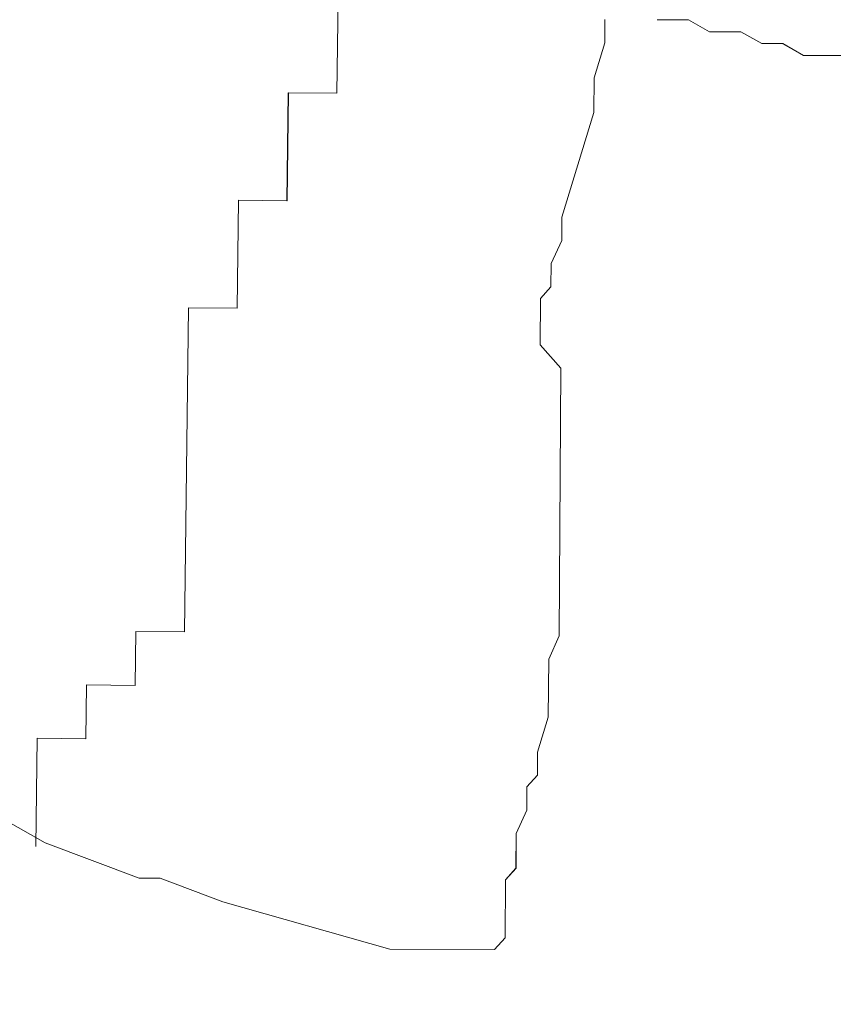
# Model space of a CAD drawing. Units: inches. Extents: x -466983 to 1020, y 324 to 318697.
# Tile 74 of 97: x 650.415 to 652.495, y 939.297 to 941.813. Entities that reach past the tile are written whole.
import ezdxf

# ---------------------------------------------------------------- set-up
doc = ezdxf.new("R2010")
doc.units = ezdxf.units.IN
doc.header["$MEASUREMENT"] = 0
doc.layers.add('A-FLOR-PATT', color=252, linetype='Continuous', lineweight=13)
doc.layers.add('A-FURN', color=8, linetype='Continuous', lineweight=18)

# ---------------------------------------------------------------- blocks, each defined once
blk = doc.blocks.new('L Shaped Sofa')
at = {"ltscale": 2}
for p, q in [((2404.3966, 749.626), (2404.4457, 749.68)), ((2404.4457, 749.68), (2404.9336, 749.6777)), ((2404.9336, 749.6777), (2405.713, 749.4572)), ((2404.3949, 749.3549), (2404.3966, 749.626)), ((2405.713, 749.4572), (2406.0051, 749.3474)), ((2404.3458, 749.3009), (2404.3949, 749.3549)), ((2406.0051, 749.3474), (2406.1027, 749.3469)), ((2406.1027, 749.3469), (2406.5409, 749.1822)), ((2404.3448, 749.1383), (2404.3458, 749.3009)), ((2406.5409, 749.1822), (2406.7354, 749.0728)), ((2406.5785, 748.695), (2406.5847, 749.1988)), ((2404.2953, 749.0301), (2404.3448, 749.1383)), ((2404.2947, 748.9217), (2404.2953, 749.0301)), ((2404.2455, 748.8677), (2404.2947, 748.9217)), ((2404.2449, 748.7592), (2404.2455, 748.8677)), ((2404.1951, 748.5968), (2404.2449, 748.7592)), ((2406.3486, 748.4458), (2406.3517, 748.6977)), ((2406.3517, 748.6977), (2406.5785, 748.695)), ((2404.1934, 748.3257), (2404.1951, 748.5968)), ((2406.1187, 748.1967), (2406.1218, 748.4486)), ((2406.1218, 748.4486), (2406.3486, 748.4458)), ((2404.144, 748.2175), (2404.1934, 748.3257)), ((2404.1363, 746.9706), (2404.144, 748.2175)), ((2405.8734, 746.688), (2405.8919, 748.1994)), ((2405.8919, 748.1994), (2406.1187, 748.1967)), ((2404.2333, 746.8617), (2404.1363, 746.9706)), ((2404.2319, 746.6448), (2404.2333, 746.8617)), ((2405.6404, 746.1869), (2405.6466, 746.6907)), ((2405.6466, 746.6907), (2405.8734, 746.688)), ((2404.1828, 746.5908), (2404.2319, 746.6448)), ((2404.1821, 746.4824), (2404.1828, 746.5908)), ((2404.1327, 746.3742), (2404.1821, 746.4824)), ((2404.132, 746.2658), (2404.1327, 746.3742)), ((2403.9826, 745.7785), (2404.132, 746.2658)), ((2405.4074, 745.6859), (2405.4136, 746.1897)), ((2405.4136, 746.1897), (2405.6404, 746.1869)), ((2403.9816, 745.6159), (2403.9826, 745.7785)), ((2405.1652, 744.4291), (2405.1806, 745.6886)), ((2405.1806, 745.6886), (2405.4074, 745.6859)), ((2403.9319, 745.4534), (2403.9816, 745.6159)), ((2402.6147, 745.5138), (2403.0051, 745.512)), ((2403.0051, 745.512), (2403.1023, 745.4573)), ((2403.1023, 745.4573), (2403.1999, 745.4569)), ((2403.1999, 745.4569), (2403.2972, 745.4022)), ((2403.9312, 745.345), (2403.9319, 745.4534)), ((2403.2972, 745.4022), (2403.4436, 745.4015)), ((2403.4436, 745.4015), (2403.5408, 745.3468)), ((2403.5408, 745.3468), (2403.6872, 745.3462))]:
    blk.add_line(p, q, dxfattribs=at)

msp = doc.modelspace()

# ---------------------------------------------------------------- hatches: boundary and pattern name
at = {"layer": 'A-FLOR-PATT', "transparency": 33554572}
h = msp.add_hatch(dxfattribs=at)
h.set_pattern_fill('ANSI37', color=256, scale=30)
h.set_pattern_definition([(45, (-1212.4137, -290.035), (-2.6516504, 2.6516504), []), (135, (-1212.4137, -290.035), (-2.6516504, -2.6516504), [])])
h.paths.add_polyline_path([(901.8057, 1075.9377), (900.6144, 1075.9377), (900.6144, 1065.3856), (899.391, 1065.3856), (898.0911, 1065.3856), (892.8356, 1058.7098, -0.258377), (892.1875, 1058.3509), (879.9848, 1058.3509, -0.20177), (879.4382, 1058.5808), (874.0812, 1065.3856), (872.7813, 1065.3856), (871.5579, 1065.3856), (871.5579, 1075.9377), (813.8057, 1075.9377), (813.8057, 1044.7922), (832.3947, 1044.7922, -0.394795), (848.6602, 1028.5356), (848.6602, 1009.9377), (901.8057, 1009.9377), (901.8057, 1015.9377), (901.3057, 1015.9377), (871.3057, 1015.9377), (871.3057, 1017.2502), (871.3344, 1017.2502, -0.401453), (901.3057, 1045.9377), (901.8057, 1045.9377)])
edge = h.paths.add_edge_path(flags=16)
edge.add_line((847.7731, 1068.9486), (847.7731, 1073.7088))
edge.add_arc((849.2269, 1073.7088), 1.4538, 90, 180, ccw=False)
edge.add_line((849.2269, 1075.1627), (864.4921, 1075.1627))
edge.add_arc((864.4921, 1073.7088), 1.4538, 0, 90, ccw=False)
edge.add_line((865.9459, 1073.7088), (865.9459, 1069.0035))
edge.add_arc((832.6447, 1068.9761), 33.3012, -20.61234, 0.04725, ccw=False)
edge.add_ellipse((856.8595, 1058.48), major_axis=(0, 10.2131), ratio=0.6859192, start_angle=100.00884, end_angle=259.99116, ccw=False)
edge.add_arc((881.0742, 1068.9761), 33.3012, 180.04725, 200.61234, ccw=False)
h.paths.add_polyline_path([(853.1456, 1066.4815), (853.1456, 1066.4534), (853.1463, 1066.4534, 0.433107), (852.9166, 1066.6849), (852.9166, 1066.4534), (853.1456, 1066.4534), (853.1456, 1066.4815), (853.088, 1066.6122, 0.697939), (852.6995, 1066.4534), (852.7003, 1066.4534), (852.7003, 1066.4815), (852.9166, 1067.0012), (852.9166, 1066.6849, -0.396254)], flags=0)
h.paths.add_polyline_path([(861.0187, 1066.4815), (861.0187, 1066.4534), (861.0194, 1066.4534, 0.416404), (860.8024, 1066.6849), (860.8024, 1066.4534), (861.0187, 1066.4534), (861.0187, 1066.4815), (860.9672, 1066.6053, 0.713344), (860.5726, 1066.4534), (860.5734, 1066.4534), (860.5734, 1066.4815), (860.8024, 1067.0012), (860.8024, 1066.6849, -0.379973)], flags=0)
edge = h.paths.add_edge_path(flags=0)
edge.add_spline(control_points=[(861.1298, 1065.7855), (861.4661, 1065.2478), (861.6134, 1065.0161), (861.9833, 1064.3736), (862.1924, 1063.9443), (862.5614, 1063.0391), (862.7212, 1062.5633), (862.9865, 1061.5781), (863.092, 1061.0689), (863.2452, 1060.031), (863.293, 1059.5025), (863.3295, 1058.4409), (863.3181, 1057.9078), (863.2366, 1056.8518), (863.1664, 1056.3289), (862.9695, 1055.308), (862.8427, 1054.8099), (862.5365, 1053.8522), (862.3571, 1053.3927), (861.9514, 1052.5249), (861.7251, 1052.1166), (861.233, 1051.3622), (860.9672, 1051.0162), (860.4048, 1050.3949), (860.1082, 1050.1197), (859.4937, 1049.6461), (859.1758, 1049.4476), (858.5276, 1049.1299), (858.1973, 1049.0107), (857.5315, 1048.8518), (857.1959, 1048.8121), (856.5249, 1048.812), (856.1894, 1048.8515), (855.5236, 1049.0101), (855.1933, 1049.1291), (854.545, 1049.4465), (854.2271, 1049.6449), (853.6124, 1050.1183), (853.3158, 1050.3933), (852.7533, 1051.0143), (852.4874, 1051.3602), (851.9952, 1052.1144), (851.7688, 1052.5225), (851.3629, 1053.3902), (851.1834, 1053.8496), (850.877, 1054.8071), (850.7501, 1055.3051), (850.553, 1056.326), (850.4827, 1056.8488), (850.401, 1057.9048), (850.3895, 1058.4379), (850.4257, 1059.4995), (850.4734, 1060.0281), (850.6265, 1061.066), (850.7318, 1061.5753), (850.9969, 1062.5605), (851.1567, 1063.0365), (851.5254, 1063.9418), (851.7345, 1064.3712), (852.1056, 1065.0164), (852.2544, 1065.2503), (852.6082, 1065.7335)], knot_values=[3.915332, 3.915332, 3.915332, 3.915332, 4.013468, 4.013468, 4.175532, 4.175532, 4.337596, 4.337596, 4.49966, 4.49966, 4.661724, 4.661724, 4.823788, 4.823788, 4.985852, 4.985852, 5.147916, 5.147916, 5.30998, 5.30998, 5.472044, 5.472044, 5.634109, 5.634109, 5.796173, 5.796173, 5.958237, 5.958237, 6.120301, 6.120301, 6.282365, 6.282365, 6.444429, 6.444429, 6.606493, 6.606493, 6.768557, 6.768557, 6.930621, 6.930621, 7.092685, 7.092685, 7.254749, 7.254749, 7.416813, 7.416813, 7.578878, 7.578878, 7.740942, 7.740942, 7.903006, 7.903006, 8.06507, 8.06507, 8.227134, 8.227134, 8.389198, 8.389198, 8.551262, 8.551262, 8.65037, 8.65037, 8.65037, 8.65037], degree=3, periodic=0)
edge.add_line((852.6421, 1065.7855), (861.1298, 1065.7855))
edge = h.paths.add_edge_path(flags=0)
edge.add_ellipse((856.8496, 1057.7432), major_axis=(0, 7.7921), ratio=0.687861, start_angle=0, end_angle=360)
h.paths.add_polyline_path([(848.8634, 1069.3891), (848.8634, 1073.9605, -0.414214), (849.9538, 1075.0508), (863.7652, 1075.0508, -0.414214), (864.8555, 1073.9605), (864.8555, 1069.3891, -0.388936), (864.5237, 1069.027, -0.043561), (849.1953, 1069.027, -0.388936)], flags=0)
h.paths.add_polyline_path([(853.1006, 1068.1122, -1), (852.6775, 1068.1122, -1)], flags=0)
edge = h.paths.add_edge_path(flags=0)
edge.add_ellipse((856.8595, 1057.3378), major_axis=(0, 2.207), ratio=0.657164, start_angle=0, end_angle=360)
h.paths.add_polyline_path([(861.0415, 1068.1122, -1), (860.6184, 1068.1122, -1)], flags=0)
edge = h.paths.add_edge_path()
edge.add_line((573.9537, 1057.3412), (573.9537, 1075.9377))
edge.add_line((573.9537, 1075.9377), (558.7308, 1075.9377))
edge.add_line((558.7308, 1075.9377), (558.7308, 1065.3856))
edge.add_line((558.7308, 1065.3856), (557.5074, 1065.3856))
edge.add_line((557.5074, 1065.3856), (556.2075, 1065.3856))
edge.add_line((556.2075, 1065.3856), (550.952, 1058.7098))
edge.add_arc((550.3039, 1059.1155), 0.7646, 270, 327.9483, ccw=False)
edge.add_line((550.3039, 1058.3509), (538.1012, 1058.3509))
edge.add_arc((538.1012, 1059.1155), 0.7646, 224.3704, 270, ccw=False)
edge.add_line((537.5546, 1058.5808), (532.1976, 1065.3856))
edge.add_line((532.1976, 1065.3856), (530.8977, 1065.3856))
edge.add_line((530.8977, 1065.3856), (529.6743, 1065.3856))
edge.add_line((529.6743, 1065.3856), (529.6743, 1075.9377))
edge.add_line((529.6743, 1075.9377), (520.8057, 1075.9377))
edge.add_line((520.8057, 1075.9377), (520.8057, 1045.9377))
edge.add_line((520.8057, 1045.9377), (521.3057, 1045.9377))
edge.add_arc((521.3057, 1015.9377), 30, 2.50749, 90, ccw=False)
edge.add_line((551.277, 1017.2502), (551.3057, 1017.2502))
edge.add_line((551.3057, 1017.2502), (551.3057, 1015.9377))
edge.add_line((551.3057, 1015.9377), (520.8057, 1015.9377))
edge.add_line((520.8057, 1015.9377), (520.8057, 1009.9377))
edge.add_line((520.8057, 1009.9377), (559.1913, 1010.4022))
edge.add_arc((559.1913, 1011.856), 1.4538, 180, 270, ccw=False)
edge.add_line((557.7375, 1011.856), (557.7375, 1016.5613))
edge.add_arc((591.0386, 1016.5888), 33.3012, 159.38766, 180.04725, ccw=False)
edge.add_ellipse((566.8239, 1027.0848), major_axis=(0, 10.2131), ratio=0.6859192, start_angle=280.00884, end_angle=439.99116, ccw=False)
edge.add_arc((542.6091, 1016.5888), 33.3012, 0.04725, 20.61234, ccw=False)
edge.add_line((575.9103, 1016.6162), (575.9103, 1011.856))
edge.add_arc((574.4565, 1011.856), 1.4538, -90, 0, ccw=False)
edge.add_line((574.4565, 1010.4022), (608.8057, 1009.9377))
edge.add_line((608.8057, 1009.9377), (608.8057, 1041.0857))
edge.add_line((608.8057, 1041.0857), (590.2179, 1041.0857))
edge.add_arc((590.775, 1057.9074), 16.8309, 181.92775, 268.10321, ccw=False)
edge = h.paths.add_edge_path()
edge.add_ellipse((494.2443, 583.6204), major_axis=(0, 10.2131), ratio=0.6859192, start_angle=280.00884, end_angle=439.99116, ccw=False)
edge.add_arc((470.0296, 573.1243), 33.3012, 0.04725, 20.61234, ccw=False)
edge.add_line((503.3307, 573.1518), (503.3307, 568.3916))
edge.add_arc((501.8769, 568.3916), 1.4538, -90, 0, ccw=False)
edge.add_line((501.8769, 566.9377), (539.8057, 566.9377))
edge.add_line((539.8057, 566.9377), (539.8057, 572.9377))
edge.add_line((539.8057, 572.9377), (539.3057, 572.9377))
edge.add_line((539.3057, 572.9377), (509.3057, 572.9377))
edge.add_line((509.3057, 572.9377), (509.3057, 574.2502))
edge.add_line((509.3057, 574.2502), (509.3344, 574.2502))
edge.add_arc((539.3057, 572.9377), 30, 90, 177.49251, ccw=False)
edge.add_line((539.3057, 602.9377), (539.8057, 602.9377))
edge.add_line((539.8057, 602.9377), (539.8057, 626.9377))
edge.add_line((539.8057, 626.9377), (531.7718, 626.9377))
edge.add_line((531.7718, 626.9377), (531.7718, 616.3856))
edge.add_line((531.7718, 616.3856), (530.5484, 616.3856))
edge.add_line((530.5484, 616.3856), (529.2485, 616.3856))
edge.add_line((529.2485, 616.3856), (523.7105, 609.3509))
edge.add_line((523.7105, 609.3509), (510.7766, 609.3509))
edge.add_line((510.7766, 609.3509), (505.2386, 616.3856))
edge.add_line((505.2386, 616.3856), (503.9387, 616.3856))
edge.add_line((503.9387, 616.3856), (502.7153, 616.3856))
edge.add_line((502.7153, 616.3856), (502.7153, 626.9377))
edge.add_line((502.7153, 626.9377), (481.6983, 626.9377))
edge.add_line((481.6983, 626.9377), (481.6983, 610.995))
edge.add_arc((467.2703, 611.4728), 14.4359, 271.92775, 358.10321, ccw=False)
edge.add_line((467.7559, 597.0451), (451.8057, 597.0451))
edge.add_line((451.8057, 597.0451), (451.8057, 584.4035))
edge.add_line((451.8057, 584.4035), (451.8057, 566.9377))
edge.add_line((451.8057, 566.9377), (486.6117, 566.9377))
edge.add_arc((486.6117, 568.3916), 1.4538, 180, 270, ccw=False)
edge.add_line((485.1579, 568.3916), (485.1579, 573.0969))
edge.add_arc((518.4591, 573.1243), 33.3012, 159.38766, 180.04725, ccw=False)
h.paths.add_polyline_path([(836.2609, 1020.7328), (879.8898, 1020.7328), (879.8898, 1039.3902), (836.2609, 1039.3902)], flags=25)
h.paths.add_polyline_path([(549.9851, 1036.7492), (593.614, 1036.7492), (593.614, 1055.4065), (549.9851, 1055.4065)], flags=24)
h.paths.add_polyline_path([(475.123, 595.5959), (518.752, 595.5959), (518.752, 614.2532), (475.123, 614.2532)], flags=24)
h = msp.add_hatch(dxfattribs=at)
h.set_pattern_fill('ANSI37', color=256, scale=20)
h.set_pattern_definition([(45, (-1212.4137, -290.035), (-1.767767, 1.767767), []), (135, (-1212.4137, -290.035), (-1.767767, -1.767767), [])])
h.paths.add_polyline_path([(809.8057, 870.9377), (809.8057, 888.1519), (806.9985, 888.1519), (802.6624, 888.1519), (789.3832, 888.1519), (786.2846, 888.1519, -0.414214), (785.4991, 888.9374), (785.4991, 900.1959), (785.4991, 908.4696, -0.414214), (786.8082, 909.7787, -0.414214), (785.4991, 911.0878), (785.4991, 929.1015, -0.414214), (786.8082, 930.4106, -0.414214), (785.4991, 931.7197), (785.4991, 931.9039, -0.414214), (784.19, 930.5948), (766.7223, 930.5948, -0.412359), (765.4132, 931.8956, -0.413741), (764.1145, 930.5782), (744.5781, 930.422, -0.416556), (743.7864, 931.2075), (743.7864, 933.5153), (742.2154, 933.5153), (742.2154, 952.024, -0.001344), (743.7864, 952.1998), (743.7864, 953.9377), (678.5915, 953.9377), (678.5915, 951.1305), (678.5915, 946.7945), (678.5915, 933.5153), (678.5915, 930.4166, -0.414214), (677.806, 929.6312), (666.5475, 929.6312), (658.2738, 929.6312, -0.414214), (656.9647, 930.9403, -0.414214), (655.6556, 929.6312), (637.6419, 929.6312, -0.414214), (636.3328, 930.9403, -0.414214), (635.0237, 929.6312), (634.8395, 929.6312, -0.414214), (636.1486, 928.322), (636.1486, 910.8544, -0.412359), (634.8478, 909.5452, -0.413741), (636.1653, 908.2466), (636.3214, 888.7102, -0.416556), (635.5359, 887.9184), (633.2281, 887.9184), (633.2281, 886.3475), (614.7194, 886.3475, -0.001344), (614.5436, 887.9184), (612.8057, 887.9184), (612.8057, 834.9377), (612.8057, 752.9377), (612.8057, 748.9377), (612.8057, 697.9377), (654.8057, 697.9377), (654.8057, 701.9377), (715.8057, 701.9377), (715.8057, 737.4353), (774.2918, 737.4353), (774.2918, 795.9377), (809.8057, 795.9377)])
h.paths.add_polyline_path([(679.2761, 849.5757, 0.102523), (682.1475, 849.2608, -0.080461), (694.5428, 849.7725, -0.283899), (694.4822, 849.0082, 0.136605), (694.4068, 848.8103, -0.030441), (694.5428, 846.8929), (694.5428, 842.6198), (694.5428, 838.3466, -0.028219), (694.4246, 836.5684), (694.425, 836.5684, 0.196187), (694.4456, 836.2708, -0.302897), (694.5428, 835.467, -0.080461), (682.1475, 835.9787, 0.102523), (679.2761, 835.6638, -0.58611), (678.6457, 836.0169), (678.6457, 849.2227, -0.58611)], flags=16)
h.paths.add_polyline_path([(679.5173, 848.6515, 0.699597), (679.476, 848.6342, 1.20716), (679.1935, 848.7422, 0.010621)], flags=0)
h.paths.add_polyline_path([(679.4923, 836.5608, -0.013798), (679.9178, 836.6594, -0.071703), (682.8533, 837.1434, -0.165743), (682.1665, 839.1006), (682.1665, 842.6094), (682.1665, 846.0603, -0.240616), (683.4733, 848.6767, -0.068263), (693.9295, 849.0082), (693.7875, 848.7083), (693.7875, 849.0228, 0.067332), (683.4733, 848.6767, 0.240616), (682.1665, 846.0603), (682.1665, 842.6094), (682.1665, 839.1006, 0.23459), (683.461, 836.5513, 0.068093), (693.7875, 836.1955), (693.7875, 836.5104), (693.9296, 836.2102, -0.077215), (682.2421, 836.7815, 0.086627), (679.5283, 836.5701, -0.628402), (679.5029, 836.5735), (679.5029, 836.6071, 0.910458)], flags=0)
h.paths.add_polyline_path([(679.476, 848.6364), (679.2069, 848.647), (679.2069, 836.5718, 0.913566), (679.3645, 836.5861), (679.476, 836.5824)], flags=0)
h.paths.add_polyline_path([(679.2761, 829.8604, 0.102523), (682.1475, 829.5455, -0.080461), (694.5428, 830.0572, -0.283899), (694.4822, 829.2929, 0.136605), (694.4068, 829.095, -0.030441), (694.5428, 827.1776), (694.5428, 822.9045), (694.5428, 818.6314, -0.028219), (694.4246, 816.8531), (694.425, 816.8532, 0.196187), (694.4456, 816.5555, -0.302897), (694.5428, 815.7517, -0.080461), (682.1475, 816.2635, 0.102523), (679.2761, 815.9485, -0.58611), (678.6457, 816.3016), (678.6457, 829.5074, -0.58611)], flags=16)
h.paths.add_polyline_path([(679.5173, 828.9362, 0.699597), (679.476, 828.9189, 1.20716), (679.1935, 829.0269, 0.010621)], flags=0)
h.paths.add_polyline_path([(679.4923, 816.8456, -0.013798), (679.9178, 816.9441, -0.071703), (682.8533, 817.4281, -0.165743), (682.1665, 819.3853), (682.1665, 822.8941), (682.1665, 826.345, -0.240616), (683.4733, 828.9614, -0.068263), (693.9295, 829.2929), (693.7875, 828.9931), (693.7875, 829.3076, 0.067332), (683.4733, 828.9614, 0.240616), (682.1665, 826.345), (682.1665, 822.8941), (682.1665, 819.3853, 0.23459), (683.461, 816.836, 0.068093), (693.7875, 816.4802), (693.7875, 816.7952), (693.9296, 816.4949, -0.077215), (682.2421, 817.0662, 0.086627), (679.5283, 816.8549, -0.628402), (679.5029, 816.8582), (679.5029, 816.8918, 0.910458)], flags=0)
h.paths.add_polyline_path([(679.476, 828.9211), (679.2069, 828.9317), (679.2069, 816.8565, 0.913566), (679.3645, 816.8708), (679.476, 816.8671)], flags=0)
h.paths.add_polyline_path([(679.2761, 810.1451, 0.102523), (682.1475, 809.8302, -0.080461), (694.5428, 810.342, -0.3023), (694.4466, 809.5394, 0.10023), (694.4058, 809.3878, -0.03057), (694.5428, 807.4623), (694.5428, 803.1892), (694.5428, 798.9161, -0.03057), (694.4058, 796.9906, 0.10023), (694.4466, 796.839, -0.3023), (694.5428, 796.0365, -0.080461), (682.1475, 796.5482, 0.102523), (679.2761, 796.2333, -0.58611), (678.6457, 796.5863), (678.6457, 809.7921, -0.58611)], flags=16)
h.paths.add_polyline_path([(679.5173, 809.2417, 0.699597), (679.476, 809.2244, 1.20716), (679.1935, 809.3324, 0.010621)], flags=0)
h.paths.add_polyline_path([(679.4923, 797.151, -0.013798), (679.9178, 797.2496, -0.071703), (682.8533, 797.7336, -0.165743), (682.1665, 799.6908), (682.1665, 803.1996), (682.1665, 806.6505, -0.239349), (683.461, 809.2577, -0.072465), (694.4468, 809.5405, 0.197932), (694.425, 809.2405), (693.7875, 809.2985), (693.7875, 809.6135, 0.068093), (683.461, 809.2577, 0.239349), (682.1665, 806.6505), (682.1665, 803.1996), (682.1665, 799.6908, 0.235854), (683.4733, 797.1323, 0.067332), (693.7875, 796.7861), (693.7875, 797.1006), (694.425, 797.1586, 0.197932), (694.4468, 796.8586, -0.080419), (682.1557, 797.3795, 0.083867), (679.5283, 797.1603, -0.628402), (679.5029, 797.1637), (679.5029, 797.1973, 0.910458)], flags=0)
h.paths.add_polyline_path([(679.2069, 809.2372), (679.2069, 797.162, 0.913566), (679.3645, 797.1763), (679.476, 797.1726), (679.476, 809.2266)], flags=0)
h.paths.add_polyline_path([(695.3643, 853.2989), (728.2231, 853.2989), (728.2231, 771.1519), (695.3643, 771.1519)], flags=16)
h.paths.add_polyline_path([(696.0215, 852.6417), (727.5659, 852.6417), (727.5659, 771.809), (696.0215, 771.809)], flags=0)
h.paths.add_polyline_path([(679.2761, 788.7869, 0.102523), (682.1475, 788.472, -0.080461), (694.5428, 788.9837, -0.3023), (694.4466, 788.1812, 0.10023), (694.4058, 788.0296, -0.03057), (694.5428, 786.1041), (694.5428, 781.831), (694.5428, 777.5578, -0.03057), (694.4058, 775.6323, 0.10023), (694.4466, 775.4808, -0.3023), (694.5428, 774.6782, -0.080461), (682.1475, 775.19, 0.102523), (679.2761, 774.875, -0.58611), (678.6457, 775.2281), (678.6457, 788.4339, -0.58611)], flags=16)
h.paths.add_polyline_path([(679.5173, 787.8834, 0.699597), (679.476, 787.8662, 1.20716), (679.1935, 787.9742, 0.010621)], flags=0)
h.paths.add_polyline_path([(679.4923, 775.7928, -0.013798), (679.9178, 775.8914, -0.071703), (682.8533, 776.3753, -0.165743), (682.1665, 778.3325), (682.1665, 781.8414), (682.1665, 785.2922, -0.239349), (683.461, 787.8995, -0.072465), (694.4468, 788.1823, 0.197932), (694.425, 787.8823), (693.7875, 787.9403), (693.7875, 788.2553, 0.068093), (683.461, 787.8995, 0.239349), (682.1665, 785.2922), (682.1665, 781.8414), (682.1665, 778.3325, 0.235854), (683.4733, 775.7741, 0.067332), (693.7875, 775.4279), (693.7875, 775.7424), (694.425, 775.8004, 0.197932), (694.4468, 775.5004, -0.080419), (682.1557, 776.0212, 0.083867), (679.5283, 775.8021, -0.628402), (679.5029, 775.8054), (679.5029, 775.8391, 0.910458)], flags=0)
h.paths.add_polyline_path([(679.2069, 787.8789), (679.2069, 775.8038, 0.913566), (679.3645, 775.818), (679.476, 775.8144), (679.476, 787.8684)], flags=0)
h.paths.add_polyline_path([(704.641, 854.1204, -0.080461), (705.1527, 866.5157, 0.102523), (704.8378, 869.3871, -0.58611), (705.1908, 870.0174), (718.3966, 870.0174, -0.58611), (718.7496, 869.3871, 0.102523), (718.4347, 866.5157, -0.080461), (718.9465, 854.1204, -0.3023), (718.1439, 854.2166, 0.10023), (717.9924, 854.2574, -0.03057), (716.0668, 854.1204), (711.7937, 854.1204), (707.5206, 854.1204, -0.03057), (705.5951, 854.2574, 0.10023), (705.4435, 854.2166, -0.3023)], flags=16)
h.paths.add_polyline_path([(717.8462, 869.1459, 0.699597), (717.8289, 869.1872, 1.20716), (717.9369, 869.4697, 0.010621)], flags=0)
h.paths.add_polyline_path([(705.4631, 854.2164, -0.080419), (705.984, 866.5074, 0.083867), (705.7648, 869.1349, -0.628402), (705.7682, 869.1603), (705.8018, 869.1603, 0.910458), (705.7555, 869.1709, -0.013798), (705.8541, 868.7454, -0.071703), (706.3381, 865.8099, -0.165743), (708.2953, 866.4967), (711.8041, 866.4967), (715.255, 866.4967, -0.239349), (717.8622, 865.2022, -0.072465), (718.145, 854.2164, 0.197932), (717.845, 854.2382), (717.903, 854.8757), (718.218, 854.8757, 0.068093), (717.8622, 865.2022, 0.239349), (715.255, 866.4967), (711.8041, 866.4967), (708.2953, 866.4967, 0.235854), (705.7368, 865.1898, 0.067332), (705.3906, 854.8757), (705.7051, 854.8757), (705.7631, 854.2382, 0.197932)], flags=16)
h.paths.add_polyline_path([(705.7665, 869.4563, 0.913566), (705.7808, 869.2987), (705.7771, 869.1872), (717.8311, 869.1872), (717.8417, 869.4563)], flags=0)
h.paths.add_polyline_path([(729.0446, 842.6198), (729.0446, 846.8929, -0.03057), (729.1817, 848.8184, 0.10023), (729.1408, 848.9699, -0.3023), (729.0446, 849.7725, -0.080461), (741.4399, 849.2608, 0.102523), (744.3113, 849.5757, -0.58611), (744.9417, 849.2227), (744.9417, 836.0169, -0.58611), (744.3113, 835.6638, 0.102523), (741.4399, 835.9787, -0.080461), (729.0446, 835.467, -0.3023), (729.1408, 836.2696, 0.10023), (729.1817, 836.4211, -0.03057), (729.0446, 838.3466)], flags=16)
h.paths.add_polyline_path([(744.1115, 836.5846, 1.20716), (744.3939, 836.4766, 0.010621), (744.0701, 836.5673, 0.699597)], flags=0)
h.paths.add_polyline_path([(729.1407, 836.2684, 0.197932), (729.1624, 836.5684), (729.7999, 836.5104), (729.7999, 836.1955, 0.068093), (740.1264, 836.5513, 0.239349), (741.4209, 839.1585), (741.4209, 842.6094), (741.4209, 846.1182, 0.235854), (740.1141, 848.6767, 0.067332), (729.7999, 849.0228), (729.7999, 848.7083), (729.1624, 848.6503, 0.197932), (729.1407, 848.9504, -0.080419), (741.4317, 848.4295, 0.083867), (744.0591, 848.6486, -0.628402), (744.0845, 848.6453), (744.0845, 848.6117, 0.910458), (744.0951, 848.6579, -0.013798), (743.6696, 848.5594, -0.071703), (740.7341, 848.0754, -0.165743), (741.4209, 846.1182), (741.4209, 842.6094), (741.4209, 839.1585, -0.239349), (740.1264, 836.5513, -0.072465)], flags=0)
h.paths.add_polyline_path([(729.0446, 830.0572, -0.080461), (741.4399, 829.5455, 0.102523), (744.3113, 829.8604, -0.58611), (744.9417, 829.5074), (744.9417, 816.3016, -0.58611), (744.3113, 815.9485, 0.102523), (741.4399, 816.2635, -0.080461), (729.0446, 815.7517, -0.3023), (729.1408, 816.5543, 0.10023), (729.1817, 816.7058, -0.03057), (729.0446, 818.6314), (729.0446, 822.9045), (729.0446, 827.1776, -0.03057), (729.1817, 829.1031, 0.10023), (729.1408, 829.2547, -0.3023)], flags=16)
h.paths.add_polyline_path([(744.1115, 816.8693, 1.20716), (744.3939, 816.7613, 0.010621), (744.0701, 816.852, 0.699597)], flags=0)
h.paths.add_polyline_path([(729.1407, 829.2351, -0.080419), (741.4317, 828.7142, 0.083867), (744.0591, 828.9334, -0.628402), (744.0845, 828.93), (744.0845, 828.8964, 0.910458), (744.0951, 828.9427, -0.013798), (743.6696, 828.8441, -0.071703), (740.7341, 828.3601, -0.165743), (741.4209, 826.4029), (741.4209, 822.8941), (741.4209, 819.4432, -0.239349), (740.1264, 816.836, -0.072465), (729.1407, 816.5531, 0.197932), (729.1624, 816.8532), (729.7999, 816.7952), (729.7999, 816.4802, 0.068093), (740.1264, 816.836, 0.239349), (741.4209, 819.4432), (741.4209, 822.8941), (741.4209, 826.4029, 0.235854), (740.1141, 828.9614, 0.067332), (729.7999, 829.3076), (729.7999, 828.9931), (729.1624, 828.9351, 0.197932)], flags=16)
h.paths.add_polyline_path([(729.0446, 810.342, -0.080461), (741.4399, 809.8302, 0.102523), (744.3113, 810.1451, -0.58611), (744.9417, 809.7921), (744.9417, 796.5863, -0.58611), (744.3113, 796.2333, 0.102523), (741.4399, 796.5482, -0.080461), (729.0446, 796.0365, -0.283899), (729.1052, 796.8007, 0.136605), (729.1806, 796.9987, -0.030441), (729.0446, 798.9161), (729.0446, 803.1892), (729.0446, 807.4623, -0.028219), (729.1628, 809.2406), (729.1624, 809.2405, 0.196187), (729.1418, 809.5382, -0.302897)], flags=16)
h.paths.add_polyline_path([(744.1115, 797.1748, 1.20716), (744.3939, 797.0668, 0.010621), (744.0701, 797.1575, 0.699597)], flags=0)
h.paths.add_polyline_path([(741.3453, 809.0275, 0.086627), (744.0591, 809.2388, -0.628402), (744.0845, 809.2355), (744.0845, 809.2019, 0.910458), (744.0951, 809.2481, -0.013798), (743.6696, 809.1496, -0.071703), (740.7341, 808.6656, -0.165743), (741.4209, 806.7084), (741.4209, 803.1996), (741.4209, 799.7487, -0.240616), (740.1141, 797.1323, -0.068263), (729.658, 796.8008), (729.7999, 797.1006), (729.7999, 796.7861, 0.067332), (740.1141, 797.1323, 0.240616), (741.4209, 799.7487), (741.4209, 803.1996), (741.4209, 806.7084, 0.23459), (740.1264, 809.2577, 0.068093), (729.7999, 809.6135), (729.7999, 809.2985), (729.6578, 809.5988, -0.077215)], flags=0)
h.paths.add_polyline_path([(704.641, 770.3304, -0.283899), (705.4053, 770.2697, 0.136605), (705.6032, 770.1944, -0.030441), (707.5206, 770.3304), (711.7937, 770.3304), (716.0668, 770.3304, -0.028219), (717.8451, 770.2122), (717.845, 770.2126, 0.196187), (718.1427, 770.2331, -0.302897), (718.9465, 770.3304, -0.080461), (718.4347, 757.9351, 0.102523), (718.7496, 755.0637, -0.58611), (718.3966, 754.4333), (705.1908, 754.4333, -0.58611), (704.8378, 755.0637, 0.102523), (705.1527, 757.9351, -0.080461)], flags=16)
h.paths.add_polyline_path([(705.762, 755.3048, 0.699597), (705.7793, 755.2635, 1.20716), (705.6713, 754.9811, 0.010621)], flags=0)
h.paths.add_polyline_path([(705.4053, 769.717), (705.7051, 769.5751), (705.3906, 769.5751, 0.067332), (705.7368, 759.2609, 0.240616), (708.3532, 757.954), (711.8041, 757.954), (715.3129, 757.954, 0.23459), (717.8622, 759.2485, 0.068093), (718.218, 769.5751), (717.903, 769.5751), (718.2033, 769.7172, -0.077215), (717.632, 758.0297, 0.086627), (717.8433, 755.3159, -0.628402), (717.84, 755.2904), (717.8064, 755.2904, 0.910458), (717.8526, 755.2799, -0.013798), (717.7541, 755.7053, -0.071703), (717.2701, 758.6409, -0.165743), (715.3129, 757.954), (711.8041, 757.954), (708.3532, 757.954, -0.240616), (705.7368, 759.2609, -0.068263)], flags=0)
h.paths.add_polyline_path([(729.0446, 788.9837, -0.080461), (741.4399, 788.472, 0.102523), (744.3113, 788.7869, -0.58611), (744.9417, 788.4339), (744.9417, 775.2281, -0.58611), (744.3113, 774.875, 0.102523), (741.4399, 775.19, -0.080461), (729.0446, 774.6782, -0.283899), (729.1052, 775.4425, 0.136605), (729.1806, 775.6405, -0.030441), (729.0446, 777.5578), (729.0446, 781.831), (729.0446, 786.1041, -0.028219), (729.1628, 787.8823), (729.1624, 787.8823, 0.196187), (729.1418, 788.1799, -0.302897)], flags=16)
h.paths.add_polyline_path([(744.1115, 775.8165, 1.20716), (744.3939, 775.7086, 0.010621), (744.0701, 775.7993, 0.699597)], flags=0)
h.paths.add_polyline_path([(741.3453, 787.6692, 0.086627), (744.0591, 787.8806, -0.628402), (744.0845, 787.8773), (744.0845, 787.8437, 0.910458), (744.0951, 787.8899, -0.013798), (743.6696, 787.7913, -0.071703), (740.7341, 787.3074, -0.165743), (741.4209, 785.3502), (741.4209, 781.8414), (741.4209, 778.3905, -0.240616), (740.1141, 775.7741, -0.068263), (729.658, 775.4425), (729.7999, 775.7424), (729.7999, 775.4279, 0.067332), (740.1141, 775.7741, 0.240616), (741.4209, 778.3905), (741.4209, 781.8414), (741.4209, 785.3502, 0.23459), (740.1264, 787.8995, 0.068093), (729.7999, 788.2553), (729.7999, 787.9403), (729.6578, 788.2405, -0.077215)], flags=0)
h.paths.add_polyline_path([(744.1115, 848.6364), (744.1115, 836.5824), (744.3805, 836.5718), (744.3805, 848.647, 0.913566), (744.2229, 848.6327)], flags=0)
h.paths.add_polyline_path([(744.2229, 828.9174), (744.1115, 828.9211), (744.1115, 816.8671), (744.3805, 816.8565), (744.3805, 828.9317, 0.913566)], flags=0)
h.paths.add_polyline_path([(717.8311, 755.2635), (705.7771, 755.2635), (705.7665, 754.9945), (717.8417, 754.9945, 0.913566), (717.8274, 755.1521)], flags=0)
h.paths.add_polyline_path([(744.2229, 809.2229), (744.1115, 809.2266), (744.1115, 797.1726), (744.3805, 797.162), (744.3805, 809.2372, 0.913566)], flags=0)
h.paths.add_polyline_path([(744.1115, 787.8684), (744.1115, 775.8144), (744.3805, 775.8038), (744.3805, 787.8789, 0.913566), (744.2229, 787.8647)], flags=0)
h.paths.add_polyline_path([(678.8774, 877.1228), (737.6127, 877.1228), (737.6127, 899.5116), (678.8774, 899.5116)], flags=24)

# ---------------------------------------------------------------- linework, layer by layer
at = {"layer": 'A-FURN', "ltscale": 2}
for p, q in [((651.2343, 942.3157), (651.2258, 941.6252)), ((651.2343, 942.3157), (651.2258, 941.6252)), ((651.2343, 942.3157), (651.2258, 941.6252)), ((651.2343, 942.3157), (651.2258, 941.6252)), ((651.2343, 942.3157), (651.2258, 941.6252)), ((651.2343, 942.3157), (651.2258, 941.6252)), ((651.9108, 941.8136), (651.9104, 941.7542)), ((651.9108, 941.8136), (651.9104, 941.7542)), ((651.9108, 941.8136), (651.9104, 941.7542)), ((651.9108, 941.8136), (651.9104, 941.7542)), ((651.9108, 941.8136), (651.9104, 941.7542)), ((651.9108, 941.8136), (651.9104, 941.7542)), ((652.1248, 941.8126), (652.0445, 941.813)), ((652.1248, 941.8126), (652.0445, 941.813)), ((652.1248, 941.8126), (652.0445, 941.813)), ((652.1248, 941.8126), (652.0445, 941.813)), ((652.1248, 941.8126), (652.0445, 941.813)), ((652.1248, 941.8126), (652.0445, 941.813)), ((652.1781, 941.7826), (652.1248, 941.8126)), ((652.1781, 941.7826), (652.1248, 941.8126)), ((652.1781, 941.7826), (652.1248, 941.8126)), ((652.1781, 941.7826), (652.1248, 941.8126)), ((652.1781, 941.7826), (652.1248, 941.8126)), ((652.1781, 941.7826), (652.1248, 941.8126)), ((652.2583, 941.7823), (652.1781, 941.7826)), ((652.2583, 941.7823), (652.1781, 941.7826)), ((652.2583, 941.7823), (652.1781, 941.7826)), ((652.2583, 941.7823), (652.1781, 941.7826)), ((652.2583, 941.7823), (652.1781, 941.7826)), ((652.2583, 941.7823), (652.1781, 941.7826)), ((652.3117, 941.7523), (652.2583, 941.7823)), ((652.3117, 941.7523), (652.2583, 941.7823)), ((652.3117, 941.7523), (652.2583, 941.7823)), ((652.3117, 941.7523), (652.2583, 941.7823)), ((652.3117, 941.7523), (652.2583, 941.7823)), ((652.3117, 941.7523), (652.2583, 941.7823)), ((651.9104, 941.7542), (651.8831, 941.6651)), ((651.9104, 941.7542), (651.8831, 941.6651)), ((651.9104, 941.7542), (651.8831, 941.6651)), ((651.9104, 941.7542), (651.8831, 941.6651)), ((651.9104, 941.7542), (651.8831, 941.6651)), ((651.9104, 941.7542), (651.8831, 941.6651)), ((652.3652, 941.752), (652.3117, 941.7523)), ((652.3652, 941.752), (652.3117, 941.7523)), ((652.3652, 941.752), (652.3117, 941.7523)), ((652.3652, 941.752), (652.3117, 941.7523)), ((652.3652, 941.752), (652.3117, 941.7523)), ((652.3652, 941.752), (652.3117, 941.7523)), ((652.4185, 941.7221), (652.3652, 941.752)), ((652.4185, 941.7221), (652.3652, 941.752)), ((652.4185, 941.7221), (652.3652, 941.752)), ((652.4185, 941.7221), (652.3652, 941.752)), ((652.4185, 941.7221), (652.3652, 941.752)), ((652.4185, 941.7221), (652.3652, 941.752)), ((652.6325, 941.7211), (652.4185, 941.7221)), ((652.6325, 941.7211), (652.4185, 941.7221)), ((652.6325, 941.7211), (652.4185, 941.7221)), ((652.6325, 941.7211), (652.4185, 941.7221)), ((652.6325, 941.7211), (652.4185, 941.7221)), ((652.6325, 941.7211), (652.4185, 941.7221)), ((651.8831, 941.6651), (651.8826, 941.576)), ((651.8831, 941.6651), (651.8826, 941.576)), ((651.8831, 941.6651), (651.8826, 941.576)), ((651.8831, 941.6651), (651.8826, 941.576)), ((651.8831, 941.6651), (651.8826, 941.576)), ((651.8831, 941.6651), (651.8826, 941.576)), ((651.1015, 941.6268), (651.0981, 941.3506)), ((651.1015, 941.6268), (651.0981, 941.3506)), ((651.1015, 941.6268), (651.0981, 941.3506)), ((651.1015, 941.6268), (651.0981, 941.3506)), ((651.1015, 941.6268), (651.0981, 941.3506)), ((651.1015, 941.6268), (651.0981, 941.3506)), ((651.2258, 941.6252), (651.1015, 941.6268)), ((651.2258, 941.6252), (651.1015, 941.6268)), ((651.2258, 941.6252), (651.1015, 941.6268)), ((651.2258, 941.6252), (651.1015, 941.6268)), ((651.2258, 941.6252), (651.1015, 941.6268)), ((651.2258, 941.6252), (651.1015, 941.6268)), ((651.8826, 941.576), (651.8007, 941.3088)), ((651.8826, 941.576), (651.8007, 941.3088)), ((651.8826, 941.576), (651.8007, 941.3088)), ((651.8826, 941.576), (651.8007, 941.3088)), ((651.8826, 941.576), (651.8007, 941.3088)), ((651.8826, 941.576), (651.8007, 941.3088)), ((650.9737, 941.3521), (650.9704, 941.0759)), ((650.9737, 941.3521), (650.9704, 941.0759)), ((650.9737, 941.3521), (650.9704, 941.0759)), ((650.9737, 941.3521), (650.9704, 941.0759)), ((650.9737, 941.3521), (650.9704, 941.0759)), ((650.9737, 941.3521), (650.9704, 941.0759)), ((651.0981, 941.3506), (650.9737, 941.3521)), ((651.0981, 941.3506), (650.9737, 941.3521)), ((651.0981, 941.3506), (650.9737, 941.3521)), ((651.0981, 941.3506), (650.9737, 941.3521)), ((651.0981, 941.3506), (650.9737, 941.3521)), ((651.0981, 941.3506), (650.9737, 941.3521)), ((651.8007, 941.3088), (651.8003, 941.2494)), ((651.8007, 941.3088), (651.8003, 941.2494)), ((651.8007, 941.3088), (651.8003, 941.2494)), ((651.8007, 941.3088), (651.8003, 941.2494)), ((651.8007, 941.3088), (651.8003, 941.2494)), ((651.8007, 941.3088), (651.8003, 941.2494)), ((651.8003, 941.2494), (651.7732, 941.1901)), ((651.8003, 941.2494), (651.7732, 941.1901)), ((651.8003, 941.2494), (651.7732, 941.1901)), ((651.8003, 941.2494), (651.7732, 941.1901)), ((651.8003, 941.2494), (651.7732, 941.1901)), ((651.8003, 941.2494), (651.7732, 941.1901)), ((651.7732, 941.1901), (651.7728, 941.1306)), ((651.7732, 941.1901), (651.7728, 941.1306)), ((651.7732, 941.1901), (651.7728, 941.1306)), ((651.7732, 941.1901), (651.7728, 941.1306)), ((651.7732, 941.1901), (651.7728, 941.1306)), ((651.7732, 941.1901), (651.7728, 941.1306)), ((651.7728, 941.1306), (651.7459, 941.101)), ((651.7728, 941.1306), (651.7459, 941.101)), ((651.7728, 941.1306), (651.7459, 941.101)), ((651.7728, 941.1306), (651.7459, 941.101)), ((651.7728, 941.1306), (651.7459, 941.101)), ((651.7728, 941.1306), (651.7459, 941.101)), ((651.7459, 941.101), (651.7452, 940.9822)), ((651.7459, 941.101), (651.7452, 940.9822)), ((651.7459, 941.101), (651.7452, 940.9822)), ((651.7459, 941.101), (651.7452, 940.9822)), ((651.7459, 941.101), (651.7452, 940.9822)), ((651.7459, 941.101), (651.7452, 940.9822)), ((650.846, 941.0774), (650.8359, 940.2488)), ((650.846, 941.0774), (650.8359, 940.2488)), ((650.846, 941.0774), (650.8359, 940.2488)), ((650.846, 941.0774), (650.8359, 940.2488)), ((650.846, 941.0774), (650.8359, 940.2488)), ((650.846, 941.0774), (650.8359, 940.2488)), ((650.9704, 941.0759), (650.846, 941.0774)), ((650.9704, 941.0759), (650.846, 941.0774)), ((650.9704, 941.0759), (650.846, 941.0774)), ((650.9704, 941.0759), (650.846, 941.0774)), ((650.9704, 941.0759), (650.846, 941.0774)), ((650.9704, 941.0759), (650.846, 941.0774)), ((651.7452, 940.9822), (651.7983, 940.9225)), ((651.7452, 940.9822), (651.7983, 940.9225)), ((651.7452, 940.9822), (651.7983, 940.9225)), ((651.7452, 940.9822), (651.7983, 940.9225)), ((651.7452, 940.9822), (651.7983, 940.9225)), ((651.7452, 940.9822), (651.7983, 940.9225)), ((651.7983, 940.9225), (651.7941, 940.2389)), ((651.7983, 940.9225), (651.7941, 940.2389)), ((651.7983, 940.9225), (651.7941, 940.2389)), ((651.7983, 940.9225), (651.7941, 940.2389)), ((651.7983, 940.9225), (651.7941, 940.2389)), ((651.7983, 940.9225), (651.7941, 940.2389)), ((650.7115, 940.2503), (650.7098, 940.1122)), ((650.7115, 940.2503), (650.7098, 940.1122)), ((650.7115, 940.2503), (650.7098, 940.1122)), ((650.7115, 940.2503), (650.7098, 940.1122)), ((650.7115, 940.2503), (650.7098, 940.1122)), ((650.7115, 940.2503), (650.7098, 940.1122)), ((650.8359, 940.2488), (650.7115, 940.2503)), ((650.8359, 940.2488), (650.7115, 940.2503)), ((650.8359, 940.2488), (650.7115, 940.2503)), ((650.8359, 940.2488), (650.7115, 940.2503)), ((650.8359, 940.2488), (650.7115, 940.2503)), ((650.8359, 940.2488), (650.7115, 940.2503)), ((651.7941, 940.2389), (651.767, 940.1795)), ((651.7941, 940.2389), (651.767, 940.1795)), ((651.7941, 940.2389), (651.767, 940.1795)), ((651.7941, 940.2389), (651.767, 940.1795)), ((651.7941, 940.2389), (651.767, 940.1795)), ((651.7941, 940.2389), (651.767, 940.1795)), ((651.767, 940.1795), (651.7661, 940.0309)), ((651.767, 940.1795), (651.7661, 940.0309)), ((651.767, 940.1795), (651.7661, 940.0309)), ((651.767, 940.1795), (651.7661, 940.0309)), ((651.767, 940.1795), (651.7661, 940.0309)), ((651.767, 940.1795), (651.7661, 940.0309)), ((650.5855, 940.1137), (650.5838, 939.9756)), ((650.5855, 940.1137), (650.5838, 939.9756)), ((650.5855, 940.1137), (650.5838, 939.9756)), ((650.5855, 940.1137), (650.5838, 939.9756)), ((650.5855, 940.1137), (650.5838, 939.9756)), ((650.5855, 940.1137), (650.5838, 939.9756)), ((650.7098, 940.1122), (650.5855, 940.1137)), ((650.7098, 940.1122), (650.5855, 940.1137)), ((650.7098, 940.1122), (650.5855, 940.1137)), ((650.7098, 940.1122), (650.5855, 940.1137)), ((650.7098, 940.1122), (650.5855, 940.1137)), ((650.7098, 940.1122), (650.5855, 940.1137)), ((651.7661, 940.0309), (651.7388, 939.9419)), ((651.7661, 940.0309), (651.7388, 939.9419)), ((651.7661, 940.0309), (651.7388, 939.9419)), ((651.7661, 940.0309), (651.7388, 939.9419)), ((651.7661, 940.0309), (651.7388, 939.9419)), ((651.7661, 940.0309), (651.7388, 939.9419)), ((650.4594, 939.9771), (650.4561, 939.7009)), ((650.4594, 939.9771), (650.4561, 939.7009)), ((650.4594, 939.9771), (650.4561, 939.7009)), ((650.4594, 939.9771), (650.4561, 939.7009)), ((650.4594, 939.9771), (650.4561, 939.7009)), ((650.4594, 939.9771), (650.4561, 939.7009)), ((650.5838, 939.9756), (650.4594, 939.9771)), ((650.5838, 939.9756), (650.4594, 939.9771)), ((650.5838, 939.9756), (650.4594, 939.9771)), ((650.5838, 939.9756), (650.4594, 939.9771)), ((650.5838, 939.9756), (650.4594, 939.9771)), ((650.5838, 939.9756), (650.4594, 939.9771)), ((651.7388, 939.9419), (651.7384, 939.8824)), ((651.7388, 939.9419), (651.7384, 939.8824)), ((651.7388, 939.9419), (651.7384, 939.8824)), ((651.7388, 939.9419), (651.7384, 939.8824)), ((651.7388, 939.9419), (651.7384, 939.8824)), ((651.7388, 939.9419), (651.7384, 939.8824)), ((651.7384, 939.8824), (651.7115, 939.8528)), ((651.7384, 939.8824), (651.7115, 939.8528)), ((651.7384, 939.8824), (651.7115, 939.8528)), ((651.7384, 939.8824), (651.7115, 939.8528)), ((651.7384, 939.8824), (651.7115, 939.8528)), ((651.7384, 939.8824), (651.7115, 939.8528)), ((651.7115, 939.8528), (651.7111, 939.7934)), ((651.7115, 939.8528), (651.7111, 939.7934)), ((651.7115, 939.8528), (651.7111, 939.7934)), ((651.7115, 939.8528), (651.7111, 939.7934)), ((651.7115, 939.8528), (651.7111, 939.7934)), ((651.7115, 939.8528), (651.7111, 939.7934)), ((651.7111, 939.7934), (651.684, 939.7341)), ((651.7111, 939.7934), (651.684, 939.7341)), ((651.7111, 939.7934), (651.684, 939.7341)), ((651.7111, 939.7934), (651.684, 939.7341)), ((651.7111, 939.7934), (651.684, 939.7341)), ((651.7111, 939.7934), (651.684, 939.7341)), ((650.4801, 939.71), (650.3734, 939.77)), ((650.4801, 939.71), (650.3734, 939.77)), ((650.4801, 939.71), (650.3734, 939.77)), ((650.4801, 939.71), (650.3734, 939.77)), ((650.4801, 939.71), (650.3734, 939.77)), ((650.4801, 939.71), (650.3734, 939.77)), ((651.684, 939.7341), (651.6835, 939.6449)), ((651.684, 939.7341), (651.6835, 939.6449)), ((651.684, 939.7341), (651.6835, 939.6449)), ((651.684, 939.7341), (651.6835, 939.6449)), ((651.684, 939.7341), (651.6835, 939.6449)), ((651.684, 939.7341), (651.6835, 939.6449)), ((650.7203, 939.6197), (650.4801, 939.71)), ((650.7203, 939.6197), (650.4801, 939.71)), ((650.7203, 939.6197), (650.4801, 939.71)), ((650.7203, 939.6197), (650.4801, 939.71)), ((650.7203, 939.6197), (650.4801, 939.71)), ((650.7203, 939.6197), (650.4801, 939.71)), ((651.6835, 939.6449), (651.6565, 939.6153)), ((651.6835, 939.6449), (651.6565, 939.6153)), ((651.6835, 939.6449), (651.6565, 939.6153)), ((651.6835, 939.6449), (651.6565, 939.6153)), ((651.6835, 939.6449), (651.6565, 939.6153)), ((651.6835, 939.6449), (651.6565, 939.6153)), ((650.7738, 939.6195), (650.7203, 939.6197)), ((650.7738, 939.6195), (650.7203, 939.6197)), ((650.7738, 939.6195), (650.7203, 939.6197)), ((650.7738, 939.6195), (650.7203, 939.6197)), ((650.7738, 939.6195), (650.7203, 939.6197)), ((650.7738, 939.6195), (650.7203, 939.6197)), ((650.9339, 939.5593), (650.7738, 939.6195)), ((650.9339, 939.5593), (650.7738, 939.6195)), ((650.9339, 939.5593), (650.7738, 939.6195)), ((650.9339, 939.5593), (650.7738, 939.6195)), ((650.9339, 939.5593), (650.7738, 939.6195)), ((650.9339, 939.5593), (650.7738, 939.6195)), ((651.6565, 939.6153), (651.6556, 939.4667)), ((651.6565, 939.6153), (651.6556, 939.4667)), ((651.6565, 939.6153), (651.6556, 939.4667)), ((651.6565, 939.6153), (651.6556, 939.4667)), ((651.6565, 939.6153), (651.6556, 939.4667)), ((651.6565, 939.6153), (651.6556, 939.4667)), ((651.3612, 939.4384), (650.9339, 939.5593)), ((651.3612, 939.4384), (650.9339, 939.5593)), ((651.3612, 939.4384), (650.9339, 939.5593)), ((651.3612, 939.4384), (650.9339, 939.5593)), ((651.3612, 939.4384), (650.9339, 939.5593)), ((651.3612, 939.4384), (650.9339, 939.5593)), ((651.6556, 939.4667), (651.6287, 939.4371)), ((651.6556, 939.4667), (651.6287, 939.4371)), ((651.6556, 939.4667), (651.6287, 939.4371)), ((651.6556, 939.4667), (651.6287, 939.4371)), ((651.6556, 939.4667), (651.6287, 939.4371)), ((651.6556, 939.4667), (651.6287, 939.4371)), ((651.6287, 939.4371), (651.3612, 939.4384)), ((651.6287, 939.4371), (651.3612, 939.4384)), ((651.6287, 939.4371), (651.3612, 939.4384)), ((651.6287, 939.4371), (651.3612, 939.4384)), ((651.6287, 939.4371), (651.3612, 939.4384)), ((651.6287, 939.4371), (651.3612, 939.4384))]:
    msp.add_line(p, q, dxfattribs=at)

# ---------------------------------------------------------------- block references
at = {"layer": 'A-FURN', "xscale": 0.5482153745360612, "yscale": 0.5482153745360612, "zscale": 0.5482153745360612, "rotation": 180}
msp.add_blockref('L Shaped Sofa', (1969.7828, 1350.4232), dxfattribs=at)

doc.saveas('drawing.dxf')
